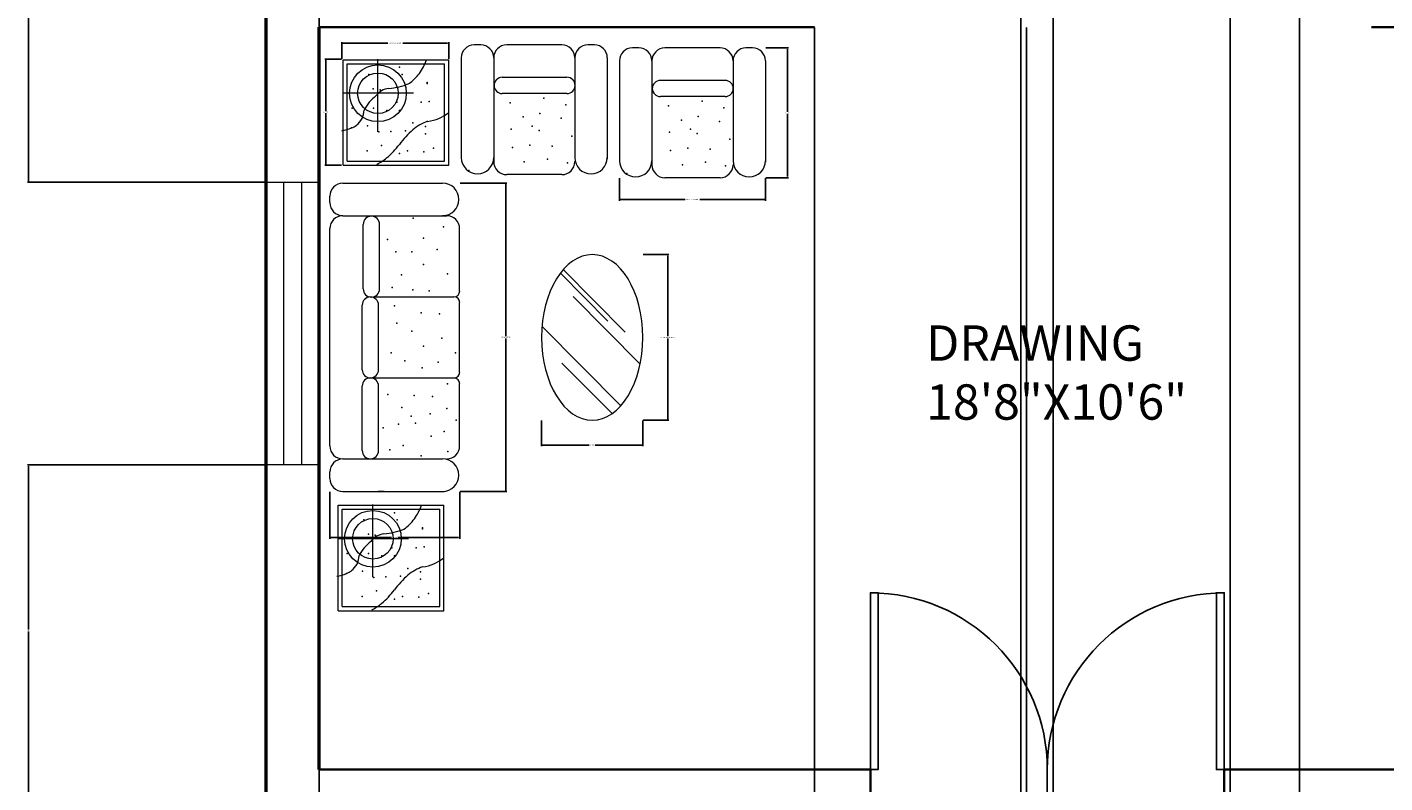
# Model space of a CAD drawing. Units: feet. Extents: x 2664 to 3060, y 1318 to 2005.
# Tile 3 of 5: x 2664 to 2894, y 1702 to 1830. Entities that reach past the tile are written whole.
import ezdxf

# ---------------------------------------------------------------- set-up
doc = ezdxf.new("R2010")
doc.units = ezdxf.units.FT
for name, color, linetype, lineweight in [('A-ANNO-DIMS', 2, 'Continuous', 18), ('A-AREA-IDEN', 109, 'Continuous', 18), ('A-WALL-EXTR', 130, 'Continuous', 50), ('DOOR', 249, 'Continuous', 25), ('FURNITURE', 240, 'Continuous', 13)]:
    doc.layers.add(name, color=color, linetype=linetype, lineweight=lineweight)
doc.layers.add('A-GLAZ', color=222, linetype='Continuous', lineweight=18, true_color=0xd4008b)
doc.layers.add('A-WALL-INTR', color=41, linetype='Continuous', lineweight=35, true_color=0xf5dd7a)
doc.styles.get("Standard").update_dxf_attribs({"font": 'arial.ttf'})
doc.dimstyles.get("Standard").update_dxf_attribs({"dimtxt": 0.18, "dimasz": 0.18, "dimexe": 0.18, "dimexo": 0.0625, "dimgap": 0.09, "dimtad": 0, "dimtih": 1, "dimtoh": 1, "dimdec": 4, "dimzin": 0, "dimdsep": 46, "dimtxsty": 'Standard', "dimcen": 0.09, "dimadec": 0, "dimazin": 0, "dimtfac": 1, "dimtdec": 4, "dimtofl": 0, "dimtmove": 0, "dimatfit": 3, "dimfxl": 1, "dimtolj": 1, "dimtzin": 0, "dimarcsym": 0})

# ---------------------------------------------------------------- blocks, each defined once
blk = doc.blocks.new('*U2')
for p, q in [((0, 0), (0, -6)), ((40, 0), (40, -6))]:
    blk.add_line(p, q)
blk.add_lwpolyline([(0, 0), (0, 40), (1.75, 40), (1.75, 0)], close=True)
blk.add_arc((0, 0), 40, 0, 90)
blk = doc.blocks.new('TABLE-END')
for p, q in [((-8.83, -9), (-8.83, 8.9)), ((-8.83, 8.9), (9.06, 8.9)), ((-8.14, -8.31), (-8.14, 8.21)), ((-8.14, 8.21), (8.38, 8.21)), ((-2.94, -3.32), (-2.94, 9)), ((8.38, -8.31), (8.38, 8.21)), ((9.06, -9), (9.06, 8.9)), ((3.1, 3.21), (-8.97, 3.21)), ((-8.83, -9), (9.06, -9)), ((-8.14, -8.31), (8.38, -8.31))]:
    blk.add_line(p, q)
for radius in [4.81, 3.44]:
    blk.add_circle((-2.94, 3.21), radius)
for centre, radius, start, end in [((-3.5, 11.98), 9.32, 324.6463, 340.6785), ((-2.19, 16.41), 12.41, 275.1129, 291.2782), ((-1.58, 10.62), 6.96, 304.0039, 324.6463), ((0.7, -2.61), 6.69, 126.4548, 153.626), ((-0.75, 0.94), 3.12, 96.1016, 144.1315), ((-8.44, 0.34), 3.14, 305.9664, 0.3439), ((-9.12, 1.28), 4.31, 293.3746, 305.9664), ((8.07, -8.93), 7.82, 109.24, 130.5005), ((4.71, 5.19), 6.79, 276.623, 309.8575), ((-9.98, 3.26), 6.46, 278.1279, 293.3746), ((12.46, -14.07), 14.57, 130.5005, 143.836), ((-9.43, 1.93), 12.54, 309.4558, 323.836), ((-7.51, -0.4), 9.52, 297.4626, 309.4558)]:
    blk.add_arc(centre, radius, start, end)
for p in [(0.71, 7.64), (-4.49, 6.42), (1.18, 6.4), (5.44, 5.05), (5.44, 4.89), (-3.72, 3.98), (-2.55, 3.81), (-7.32, 0.7), (-3.69, 0.7), (-1.43, 0.31), (0.25, 1.69), (0.71, 0.31), (4.37, 1.69), (5.75, 1.84), (3, -1.82), (-7.41, -2.67), (-4.73, -2.3), (-2.81, -3.35), (-0.75, -3.26), (1.74, -3.15), (5.12, -2.41), (5.14, -3.65), (-4.79, -6.56), (-2.35, -5.64), (2.08, -6.56), (4.83, -6.71), (6.51, -6.1), (0.72, -7.03)]:
    blk.add_point(p)
blk = doc.blocks.new('SOFA-3-SEAT')
for p, q in [((-11.01, -3.3), (-11.01, -2.2)), ((-8.81, 0), (8.12, 0)), ((-8.81, -5.51), (-4.95, -5.51)), ((-4.95, -5.51), (8.81, -5.51)), ((-11.01, -44.59), (-11.01, -7.71)), ((-5.34, -17.95), (-5.34, -6.98)), ((-2.59, -17.95), (-2.59, -6.98)), ((11.01, -18.31), (11.01, -7.71)), ((-5.51, -31.66), (-5.51, -20.69)), ((-3.58, -19.27), (10.05, -19.27)), ((-2.75, -31.66), (-2.75, -20.69)), ((11.01, -32.07), (11.01, -20.23)), ((-5.51, -45.38), (-5.51, -34.41)), ((-4.13, -33.03), (10.05, -33.03)), ((-2.75, -45.38), (-2.75, -34.41)), ((11.01, -44.59), (11.01, -34.04)), ((-8.81, -46.8), (8.12, -46.8)), ((-11.01, -50.1), (-11.01, -49)), ((-8.81, -52.3), (8.4, -52.3)), ((-2.79, -52.3), (-2.81, -52.3)), ((-1.79, -52.3), (-2.79, -52.3))]:
    blk.add_line(p, q)
for centre, radius, start, end in [((-8.81, -2.2), 2.2, 90, 180), ((8.12, -2.75), 2.75, 0, 90), ((-8.81, -3.3), 2.2, 180, 270), ((8.12, -2.75), 2.75, 270, 0), ((-8.81, -7.71), 2.2, 90, 180), ((-3.96, -6.98), 1.38, 90, 180), ((-3.96, -6.98), 1.38, 0, 90), ((8.81, -7.71), 2.2, 0, 90), ((-3.96, -17.95), 1.38, 180, 270), ((-3.96, -17.95), 1.38, 270, 0), ((10.05, -18.31), 0.963, 270, 0), ((-4.13, -20.69), 1.38, 90, 180), ((-4.13, -20.69), 1.38, 0, 90), ((10.05, -20.23), 0.963, 0, 90), ((-4.13, -31.66), 1.38, 180, 270), ((-4.13, -31.66), 1.38, 270, 0), ((10.05, -32.07), 0.963, 270, 0), ((-4.13, -34.41), 1.38, 90, 180), ((-4.13, -34.41), 1.38, 0, 90), ((10.05, -34.04), 0.963, 0, 90), ((-8.81, -44.59), 2.2, 180, 270), ((-4.13, -45.38), 1.38, 180, 270), ((-4.13, -45.38), 1.38, 270, 0), ((8.81, -44.59), 2.2, 270, 0), ((-8.81, -49), 2.2, 90, 180), ((8.12, -49.55), 2.75, 0, 90), ((-8.81, -50.1), 2.2, 180, 270), ((8.12, -49.55), 2.75, 270, 0), ((-2.76, -44.04), 8.26, 268.9725, 269.066), ((-2.75, -42.86), 9.44, 269.1265, 269.4492), ((-2.75, -44.04), 8.26, 269.411, 269.6618), ((-2.78, -44.04), 8.26, 269.9826, 270)]:
    blk.add_arc(centre, radius, start, end)
for p in [(3.15, -5.94), (8.25, -7.42), (-1.22, -9.57), (4.85, -9.35), (7.19, -11.26), (0.16, -11.65), (2.9, -11.65), (4.85, -13.8), (1.14, -15.55), (8.94, -15.36), (-0.42, -17.7), (3.09, -18.09), (5.82, -18.28), (-0.03, -20.82), (4.46, -21.98), (7.58, -22.18), (0.36, -23.74), (2.9, -25.1), (7.97, -26.27), (-0.62, -28.81), (4.85, -27.64), (10.31, -28.81), (1.73, -30.17), (4.65, -31.34), (7.38, -30.37), (8.94, -34.07), (-1.2, -35.83), (3.29, -36.02), (6.41, -36.22), (1.22, -38.06), (6.02, -39.14), (8.84, -38.21), (0.63, -40.87), (2.78, -39.55), (3.52, -40.73), (10.4, -40.21), (-1.96, -41.54), (6.18, -42.95), (8.4, -42.13), (-0.85, -45.24), (1.44, -44.5), (8.99, -45.54), (4.48, -46.28)]:
    blk.add_point(p)
blk = doc.blocks.new('TABLE-COFFEE-OVAL')
for p, q in [((2.67, 2.77), (-5.41, 10.92)), ((5.56, 0.91), (-4.93, 11.5)), ((8.13, -4.53), (-3.25, 6.96)), ((4.85, -11.6), (-8.51, 1.88)), ((3.36, -12.93), (-5.15, -4.35))]:
    blk.add_line(p, q)
at = {"extrusion": (0, 0, -1)}
blk.add_ellipse((0, 0), major_axis=(0, 14.05), ratio=0.611621, dxfattribs=at)
blk = doc.blocks.new('CHAIR-ARM')
for p, q in [((-9.08, 0), (-10.19, 0)), ((4.68, 0), (-4.68, 0)), ((10.19, 0), (9.08, 0)), ((-12.39, -2.2), (-12.39, -19.13)), ((-6.88, -2.2), (-6.88, -6.06)), ((-6.88, -2.2), (-6.88, -6.12)), ((-6.88, -2.2), (-6.88, -19.82)), ((6.88, -2.2), (6.88, -19.13)), ((12.39, -2.2), (12.39, -19.41)), ((5.54, -5.51), (-5.43, -5.51)), ((5.54, -8.26), (-5.43, -8.26)), ((4.68, -8.26), (-4.68, -8.26)), ((4.68, -22.02), (-4.68, -22.02))]:
    blk.add_line(p, q)
for centre, radius, start, end in [((-10.19, -2.2), 2.2, 90, 180), ((-9.08, -2.2), 2.2, 0, 90), ((-4.68, -2.2), 2.2, 90, 180), ((4.68, -2.2), 2.2, 0, 90), ((9.08, -2.2), 2.2, 90, 180), ((10.19, -2.2), 2.2, 0, 90), ((-5.43, -6.88), 1.38, 90, 180), ((-5.43, -6.88), 1.38, 180, 270), ((5.54, -6.88), 1.38, 0, 90), ((5.54, -6.88), 1.38, 270, 0), ((-9.63, -19.13), 2.75, 180, 270), ((-9.63, -19.13), 2.75, 270, 0), ((-4.68, -19.82), 2.2, 180, 270), ((4.68, -19.82), 2.2, 270, 0), ((9.63, -19.13), 2.75, 180, 270), ((9.63, -19.13), 2.75, 270, 0)]:
    blk.add_arc(centre, radius, start, end)
for p in [(1.63, -9.05), (-4.09, -9.81), (5.33, -10.16), (-1.86, -12.23), (-0.36, -13.79), (0.96, -11.64), (4.59, -12.46), (-3.89, -14.3), (0.81, -14.53), (6.36, -15.49), (-3.7, -17.42), (-0.77, -17.03), (3.03, -17.19), (-1.71, -19.86), (2.22, -19.41), (5.62, -20), (-11.11, -21.32)]:
    blk.add_point(p)
blk = doc.blocks.new('WINDOW-4FT')
for p, q in [((-24, 4.5), (24, 4.5)), ((-24, -4.5), (-24, 4.5)), ((24, 4.5), (24, -4.5)), ((-24, 1.5), (24, 1.5)), ((24, -1.5), (-24, -1.5)), ((24, -4.5), (-24, -4.5))]:
    blk.add_line(p, q)
blk = doc.blocks.new('*D20')
at = {"layer": 'A-ANNO-DIMS', "color": 0, "lineweight": -2, "transparency": 16777216}
for p, q in [((2717.13, 1824.69), (2717.13, 1827.53)), ((2717.31, 1827.35), (2724.94, 1827.35)), ((2735.08, 1827.35), (2727.45, 1827.35)), ((2735.26, 1824.69), (2735.26, 1827.53))]:
    blk.add_line(p, q, dxfattribs=at)
at = {"layer": 'A-ANNO-DIMS', "color": 0, "transparency": 16777216}
for points in [[(2717.31, 1827.38), (2717.31, 1827.32), (2717.13, 1827.35)], [(2735.08, 1827.38), (2735.08, 1827.32), (2735.26, 1827.35)]]:
    blk.add_solid(points, dxfattribs=at)
at = {"layer": 'Defpoints', "color": 0, "transparency": 16777216}
for p in [(2735.26, 1827.35), (2717.13, 1824.63), (2735.26, 1824.63)]:
    blk.add_point(p, dxfattribs=at)
at = {"layer": 'A-ANNO-DIMS', "color": 0, "transparency": 16777216, "insert": (2726.19, 1827.35), "char_height": 0.18, "attachment_point": 5}
blk.add_mtext('\\A1;END TABLE 18 TYP.', dxfattribs=at)
blk = doc.blocks.new('*D21')
at = {"layer": 'A-ANNO-DIMS', "color": 0, "lineweight": -2, "transparency": 16777216}
for p, q in [((2717.07, 1824.63), (2714.23, 1824.63)), ((2714.41, 1824.45), (2714.41, 1815.81)), ((2714.41, 1806.81), (2714.41, 1815.45)), ((2717.07, 1806.63), (2714.23, 1806.63))]:
    blk.add_line(p, q, dxfattribs=at)
at = {"layer": 'A-ANNO-DIMS', "color": 0, "transparency": 16777216}
for points in [[(2714.38, 1824.45), (2714.44, 1824.45), (2714.41, 1824.63)], [(2714.38, 1806.81), (2714.44, 1806.81), (2714.41, 1806.63)]]:
    blk.add_solid(points, dxfattribs=at)
at = {"layer": 'Defpoints', "color": 0, "transparency": 16777216}
for p in [(2714.41, 1824.63), (2717.13, 1824.63), (2717.13, 1806.63)]:
    blk.add_point(p, dxfattribs=at)
at = {"layer": 'A-ANNO-DIMS', "color": 0, "transparency": 16777216, "insert": (2714.41, 1815.63), "char_height": 0.18, "attachment_point": 5}
blk.add_mtext('\\A1;18 TYP.', dxfattribs=at)
blk = doc.blocks.new('*D22')
at = {"layer": 'A-ANNO-DIMS', "color": 0, "lineweight": -2, "transparency": 16777216}
for p, q in [((2764.21, 1804.45), (2764.21, 1800.62)), ((2788.99, 1804.45), (2788.99, 1800.62)), ((2764.39, 1800.8), (2775.36, 1800.8)), ((2788.81, 1800.8), (2777.84, 1800.8))]:
    blk.add_line(p, q, dxfattribs=at)
at = {"layer": 'A-ANNO-DIMS', "color": 0, "transparency": 16777216}
for points in [[(2764.39, 1800.83), (2764.39, 1800.77), (2764.21, 1800.8)], [(2788.81, 1800.83), (2788.81, 1800.77), (2788.99, 1800.8)]]:
    blk.add_solid(points, dxfattribs=at)
at = {"layer": 'Defpoints', "color": 0, "transparency": 16777216}
for p in [(2764.21, 1804.52), (2788.99, 1804.52), (2788.99, 1800.8)]:
    blk.add_point(p, dxfattribs=at)
at = {"layer": 'A-ANNO-DIMS', "color": 0, "transparency": 16777216, "insert": (2776.6, 1800.8), "char_height": 0.18, "attachment_point": 5}
blk.add_mtext('\\A1;ARMCHAIR 25 TYP.', dxfattribs=at)
blk = doc.blocks.new('*D23')
at = {"layer": 'A-ANNO-DIMS', "color": 0, "lineweight": -2, "transparency": 16777216}
for p, q in [((2789.05, 1826.54), (2792.88, 1826.54)), ((2792.7, 1826.36), (2792.7, 1815.71)), ((2792.7, 1804.7), (2792.7, 1815.35)), ((2789.05, 1804.52), (2792.88, 1804.52))]:
    blk.add_line(p, q, dxfattribs=at)
at = {"layer": 'A-ANNO-DIMS', "color": 0, "transparency": 16777216}
for points in [[(2792.67, 1826.36), (2792.73, 1826.36), (2792.7, 1826.54)], [(2792.67, 1804.7), (2792.73, 1804.7), (2792.7, 1804.52)]]:
    blk.add_solid(points, dxfattribs=at)
at = {"layer": 'Defpoints', "color": 0, "transparency": 16777216}
for p in [(2788.99, 1826.54), (2792.7, 1826.54), (2788.99, 1804.52)]:
    blk.add_point(p, dxfattribs=at)
at = {"layer": 'A-ANNO-DIMS', "color": 0, "transparency": 16777216, "insert": (2792.7, 1815.53), "char_height": 0.18, "attachment_point": 5}
blk.add_mtext('\\A1;22 TYP.', dxfattribs=at)
blk = doc.blocks.new('*D26')
at = {"layer": 'A-ANNO-DIMS', "color": 0, "lineweight": -2, "transparency": 16777216}
for p, q in [((2737.18, 1803.58), (2745.14, 1803.58)), ((2744.96, 1803.4), (2744.96, 1777.62)), ((2744.96, 1751.46), (2744.96, 1777.25)), ((2737.18, 1751.28), (2745.14, 1751.28))]:
    blk.add_line(p, q, dxfattribs=at)
at = {"layer": 'A-ANNO-DIMS', "color": 0, "transparency": 16777216}
for points in [[(2744.93, 1803.4), (2744.99, 1803.4), (2744.96, 1803.58)], [(2744.93, 1751.46), (2744.99, 1751.46), (2744.96, 1751.28)]]:
    blk.add_solid(points, dxfattribs=at)
at = {"layer": 'Defpoints', "color": 0, "transparency": 16777216}
for p in [(2737.12, 1803.58), (2744.96, 1803.58), (2737.12, 1751.28)]:
    blk.add_point(p, dxfattribs=at)
at = {"layer": 'A-ANNO-DIMS', "color": 0, "transparency": 16777216, "insert": (2744.96, 1777.43), "char_height": 0.18, "attachment_point": 5}
blk.add_mtext('\\A1;SOFA 52 TYP.', dxfattribs=at)
blk = doc.blocks.new('*D27')
at = {"layer": 'A-ANNO-DIMS', "color": 0, "lineweight": -2, "transparency": 16777216}
for p, q in [((2715.1, 1751.22), (2715.1, 1743.26)), ((2737.12, 1751.22), (2737.12, 1743.26)), ((2715.28, 1743.44), (2725.58, 1743.44)), ((2736.94, 1743.44), (2726.64, 1743.44))]:
    blk.add_line(p, q, dxfattribs=at)
at = {"layer": 'A-ANNO-DIMS', "color": 0, "transparency": 16777216}
for points in [[(2715.28, 1743.47), (2715.28, 1743.41), (2715.1, 1743.44)], [(2736.94, 1743.47), (2736.94, 1743.41), (2737.12, 1743.44)]]:
    blk.add_solid(points, dxfattribs=at)
at = {"layer": 'Defpoints', "color": 0, "transparency": 16777216}
for p in [(2715.1, 1751.28), (2737.12, 1751.28), (2737.12, 1743.44)]:
    blk.add_point(p, dxfattribs=at)
at = {"layer": 'A-ANNO-DIMS', "color": 0, "transparency": 16777216, "insert": (2726.11, 1743.44), "char_height": 0.18, "attachment_point": 5}
blk.add_mtext('\\A1;22 TYP.', dxfattribs=at)
blk = doc.blocks.new('*D28')
at = {"layer": 'A-ANNO-DIMS', "color": 0, "lineweight": -2, "transparency": 16777216}
for p, q in [((2768.26, 1791.46), (2772.59, 1791.46)), ((2772.41, 1791.28), (2772.41, 1777.6)), ((2772.41, 1763.55), (2772.41, 1777.23)), ((2768.26, 1763.37), (2772.59, 1763.37))]:
    blk.add_line(p, q, dxfattribs=at)
at = {"layer": 'A-ANNO-DIMS', "color": 0, "transparency": 16777216}
for points in [[(2772.38, 1791.28), (2772.44, 1791.28), (2772.41, 1791.46)], [(2772.38, 1763.55), (2772.44, 1763.55), (2772.41, 1763.37)]]:
    blk.add_solid(points, dxfattribs=at)
at = {"layer": 'Defpoints', "color": 0, "transparency": 16777216}
for p in [(2768.19, 1791.46), (2772.41, 1791.46), (2768.19, 1763.37)]:
    blk.add_point(p, dxfattribs=at)
at = {"layer": 'A-ANNO-DIMS', "color": 0, "transparency": 16777216, "insert": (2772.41, 1777.42), "char_height": 0.18, "attachment_point": 5}
blk.add_mtext('\\A1;COFFEE TABLE 28 TYP.', dxfattribs=at)
blk = doc.blocks.new('*D29')
at = {"layer": 'A-ANNO-DIMS', "color": 0, "lineweight": -2, "transparency": 16777216}
for p, q in [((2751.01, 1763.3), (2751.01, 1758.97)), ((2768.19, 1763.3), (2768.19, 1758.97)), ((2751.19, 1759.15), (2759.08, 1759.15)), ((2768.01, 1759.15), (2760.12, 1759.15))]:
    blk.add_line(p, q, dxfattribs=at)
at = {"layer": 'A-ANNO-DIMS', "color": 0, "transparency": 16777216}
for points in [[(2751.19, 1759.18), (2751.19, 1759.12), (2751.01, 1759.15)], [(2768.01, 1759.18), (2768.01, 1759.12), (2768.19, 1759.15)]]:
    blk.add_solid(points, dxfattribs=at)
at = {"layer": 'Defpoints', "color": 0, "transparency": 16777216}
for p in [(2751.01, 1763.37), (2768.19, 1763.37), (2768.19, 1759.15)]:
    blk.add_point(p, dxfattribs=at)
at = {"layer": 'A-ANNO-DIMS', "color": 0, "transparency": 16777216, "insert": (2759.6, 1759.15), "char_height": 0.18, "attachment_point": 5}
blk.add_mtext('\\A1;17 TYP.', dxfattribs=at)
blk = doc.blocks.new('*D41')
at = {"layer": 'A-ANNO-DIMS', "color": 0, "lineweight": -2, "transparency": 16777216}
for p, q in [((2704.22, 1875.57), (2663.82, 1875.57)), ((2664, 1875.39), (2664, 1839.85)), ((2664, 1803.95), (2664, 1839.49)), ((2704.22, 1803.77), (2663.82, 1803.77))]:
    blk.add_line(p, q, dxfattribs=at)
at = {"layer": 'A-ANNO-DIMS', "color": 0, "transparency": 16777216}
for points in [[(2663.97, 1875.39), (2664.03, 1875.39), (2664, 1875.57)], [(2663.97, 1803.95), (2664.03, 1803.95), (2664, 1803.77)]]:
    blk.add_solid(points, dxfattribs=at)
at = {"layer": 'Defpoints', "color": 0, "transparency": 16777216}
for p in [(2704.28, 1875.57), (2664, 1803.77), (2704.28, 1803.77)]:
    blk.add_point(p, dxfattribs=at)
at = {"layer": 'A-ANNO-DIMS', "color": 0, "transparency": 16777216, "insert": (2664, 1839.67), "char_height": 0.18, "attachment_point": 5}
blk.add_mtext('\\A1;71.8', dxfattribs=at)
blk = doc.blocks.new('*D42')
at = {"layer": 'A-ANNO-DIMS', "color": 0, "lineweight": -2, "transparency": 16777216}
for p, q in [((2704.22, 1755.77), (2663.82, 1755.77)), ((2664, 1755.59), (2664, 1727.85)), ((2664, 1699.75), (2664, 1727.49)), ((2704.22, 1699.57), (2663.82, 1699.57))]:
    blk.add_line(p, q, dxfattribs=at)
at = {"layer": 'A-ANNO-DIMS', "color": 0, "transparency": 16777216}
for points in [[(2663.97, 1755.59), (2664.03, 1755.59), (2664, 1755.77)], [(2663.97, 1699.75), (2664.03, 1699.75), (2664, 1699.57)]]:
    blk.add_solid(points, dxfattribs=at)
at = {"layer": 'Defpoints', "color": 0, "transparency": 16777216}
for p in [(2704.28, 1755.77), (2664, 1699.57), (2704.28, 1699.57)]:
    blk.add_point(p, dxfattribs=at)
at = {"layer": 'A-ANNO-DIMS', "color": 0, "transparency": 16777216, "insert": (2664, 1727.67), "char_height": 0.18, "attachment_point": 5}
blk.add_mtext('\\A1;56.2', dxfattribs=at)
blk = doc.blocks.new('*D48')
at = {"layer": 'A-ANNO-DIMS', "color": 0, "lineweight": -2, "transparency": 16777216}
for p, q in [((2879.53, 1619.63), (2879.53, 2005.03)), ((2879.71, 2004.85), (2929.25, 2004.85)), ((2979.35, 2004.85), (2929.81, 2004.85)), ((2979.53, 1619.63), (2979.53, 2005.03))]:
    blk.add_line(p, q, dxfattribs=at)
at = {"layer": 'A-ANNO-DIMS', "color": 0, "transparency": 16777216}
for points in [[(2879.71, 2004.88), (2879.71, 2004.82), (2879.53, 2004.85)], [(2979.35, 2004.88), (2979.35, 2004.82), (2979.53, 2004.85)]]:
    blk.add_solid(points, dxfattribs=at)
at = {"layer": 'Defpoints', "color": 0, "transparency": 16777216}
for p in [(2979.53, 2004.85), (2879.53, 1619.57), (2979.53, 1619.57)]:
    blk.add_point(p, dxfattribs=at)
at = {"layer": 'A-ANNO-DIMS', "color": 0, "transparency": 16777216, "insert": (2929.53, 2004.85), "char_height": 0.18, "attachment_point": 5}
blk.add_mtext('\\A1;100', dxfattribs=at)
blk = doc.blocks.new('*D53')
at = {"layer": 'A-ANNO-DIMS', "color": 0, "lineweight": -2, "transparency": 16777216}
for p, q in [((2797.28, 1830.01), (2797.28, 1318.11)), ((2833.28, 1830.01), (2833.28, 1318.11)), ((2797.46, 1318.29), (2815.06, 1318.29)), ((2833.1, 1318.29), (2815.5, 1318.29))]:
    blk.add_line(p, q, dxfattribs=at)
at = {"layer": 'A-ANNO-DIMS', "color": 0, "transparency": 16777216}
for points in [[(2797.46, 1318.32), (2797.46, 1318.26), (2797.28, 1318.29)], [(2833.1, 1318.32), (2833.1, 1318.26), (2833.28, 1318.29)]]:
    blk.add_solid(points, dxfattribs=at)
at = {"layer": 'Defpoints', "color": 0, "transparency": 16777216}
for p in [(2797.28, 1830.07), (2833.28, 1830.07), (2833.28, 1318.29)]:
    blk.add_point(p, dxfattribs=at)
at = {"layer": 'A-ANNO-DIMS', "color": 0, "transparency": 16777216, "insert": (2815.28, 1318.29), "char_height": 0.18, "attachment_point": 5}
blk.add_mtext('\\A1;36', dxfattribs=at)
blk = doc.blocks.new('*D54')
at = {"layer": 'A-ANNO-DIMS', "color": 0, "lineweight": -2, "transparency": 16777216}
for p, q in [((2837.78, 1868.51), (2837.78, 1318.11)), ((2867.78, 1868.51), (2867.78, 1318.11)), ((2837.96, 1318.29), (2852.56, 1318.29)), ((2867.6, 1318.29), (2853, 1318.29))]:
    blk.add_line(p, q, dxfattribs=at)
at = {"layer": 'A-ANNO-DIMS', "color": 0, "transparency": 16777216}
for points in [[(2837.96, 1318.32), (2837.96, 1318.26), (2837.78, 1318.29)], [(2867.6, 1318.32), (2867.6, 1318.26), (2867.78, 1318.29)]]:
    blk.add_solid(points, dxfattribs=at)
at = {"layer": 'Defpoints', "color": 0, "transparency": 16777216}
for p in [(2837.78, 1868.57), (2867.78, 1868.57), (2867.78, 1318.29)]:
    blk.add_point(p, dxfattribs=at)
at = {"layer": 'A-ANNO-DIMS', "color": 0, "transparency": 16777216, "insert": (2852.78, 1318.29), "char_height": 0.18, "attachment_point": 5}
blk.add_mtext('\\A1;30', dxfattribs=at)
blk = doc.blocks.new('*D55')
at = {"layer": 'A-ANNO-DIMS', "color": 0, "lineweight": -2, "transparency": 16777216}
for p, q in [((2833.28, 1830.01), (2833.28, 1318.11)), ((2837.78, 1830.01), (2837.78, 1318.11)), ((2833.46, 1318.29), (2835.27, 1318.29)), ((2837.6, 1318.29), (2835.79, 1318.29))]:
    blk.add_line(p, q, dxfattribs=at)
at = {"layer": 'A-ANNO-DIMS', "color": 0, "transparency": 16777216}
for points in [[(2833.46, 1318.32), (2833.46, 1318.26), (2833.28, 1318.29)], [(2837.6, 1318.32), (2837.6, 1318.26), (2837.78, 1318.29)]]:
    blk.add_solid(points, dxfattribs=at)
at = {"layer": 'Defpoints', "color": 0, "transparency": 16777216}
for p in [(2833.28, 1830.07), (2837.78, 1830.07), (2837.78, 1318.29)]:
    blk.add_point(p, dxfattribs=at)
at = {"layer": 'A-ANNO-DIMS', "color": 0, "transparency": 16777216, "insert": (2835.53, 1318.29), "char_height": 0.18, "attachment_point": 5}
blk.add_mtext('\\A1;4.5', dxfattribs=at)
blk = doc.blocks.new('*D59')
at = {"layer": 'A-ANNO-DIMS', "color": 0, "lineweight": -2, "transparency": 16777216}
for p, q in [((2713.28, 1488.63), (2713.28, 2005.03)), ((2713.46, 2004.85), (2772.5, 2004.85)), ((2832.1, 2004.85), (2773.06, 2004.85)), ((2832.28, 1489.53), (2832.28, 2005.03))]:
    blk.add_line(p, q, dxfattribs=at)
at = {"layer": 'A-ANNO-DIMS', "color": 0, "transparency": 16777216}
for points in [[(2713.46, 2004.88), (2713.46, 2004.82), (2713.28, 2004.85)], [(2832.1, 2004.88), (2832.1, 2004.82), (2832.28, 2004.85)]]:
    blk.add_solid(points, dxfattribs=at)
at = {"layer": 'Defpoints', "color": 0, "transparency": 16777216}
for p in [(2832.28, 2004.85), (2713.28, 1488.57), (2832.28, 1489.47)]:
    blk.add_point(p, dxfattribs=at)
at = {"layer": 'A-ANNO-DIMS', "color": 0, "transparency": 16777216, "insert": (2772.78, 2004.85), "char_height": 0.18, "attachment_point": 5}
blk.add_mtext('\\A1;119', dxfattribs=at)

msp = doc.modelspace()

# ---------------------------------------------------------------- linework, layer by layer
at = {"layer": 'A-WALL-EXTR'}
for p, q in [((2704.28, 1349.571), (2704.28, 1973.571)), ((2713.28, 1704.071), (2713.28, 1830.071))]:
    msp.add_line(p, q, dxfattribs=at)
at = {"layer": 'A-WALL-INTR'}
for p, q in [((2713.28, 1830.071), (2797.28, 1830.071)), ((2891.78, 1830.071), (2896.28, 1830.071)), ((2713.28, 1704.071), (2806.78, 1704.071)), ((2806.78, 1699.571), (2806.78, 1704.071)), ((2866.78, 1699.571), (2866.78, 1704.071)), ((2866.78, 1704.071), (2936.78, 1704.071))]:
    msp.add_line(p, q, dxfattribs=at)

# ---------------------------------------------------------------- block references
at = {"layer": 'A-GLAZ', "rotation": 89.99999999999957}
msp.add_blockref('WINDOW-4FT', (2708.78, 1779.772), dxfattribs=at)
at = {"layer": 'DOOR', "yscale": 0.7500000000000038, "zscale": 0.7500000000000038}
for p, xscale in [((2806.78, 1704.071), 0.7500000000000038), ((2866.78, 1704.071), -0.7500000000000038)]:
    msp.add_blockref('*U2', p, dxfattribs=dict(at, xscale=xscale))
at = {"layer": 'FURNITURE'}
for name, p in [('CHAIR-ARM', (2749.769, 1827.061)), ('CHAIR-ARM', (2776.599, 1826.538)), ('TABLE-END', (2726.193, 1815.632)), ('SOFA-3-SEAT', (2726.106, 1803.584)), ('TABLE-COFFEE-OVAL', (2759.601, 1777.415)), ('TABLE-END', (2725.347, 1740.034))]:
    msp.add_blockref(name, p, dxfattribs=at)

# ---------------------------------------------------------------- texts
at = {"layer": 'A-AREA-IDEN', "insert": (2816.227, 1779.457), "char_height": 6, "attachment_point": 1}
msp.add_mtext_dynamic_manual_height_columns('DRAWING \\P18\'8"X10\'6"', width=22.955, gutter_width=12.5, heights=[0], dxfattribs=at)

# ---------------------------------------------------------------- dimensions: what is measured, and where the dimension line sits
at = {"layer": 'A-ANNO-DIMS'}
for base, p1, p2, override, picture, middle in [((2832.28, 2004.851), (2713.28, 1488.571), (2832.28, 1489.471), {"dimdec": 0, "dimlfac": 1, "dimrnd": 0, "dimzin": 0, "dimdsep": 46, "dimlunit": 2}, '*D59', (2772.78, 2004.851)), ((2979.53, 2004.851), (2879.53, 1619.571), (2979.53, 1619.571), {"dimdec": 0, "dimlfac": 1, "dimrnd": 0, "dimzin": 0, "dimdsep": 46, "dimlunit": 2}, '*D48', (2929.53, 2004.851)), ((2867.78, 1318.291), (2837.78, 1868.571), (2867.78, 1868.571), {"dimdec": 0, "dimlfac": 1, "dimrnd": 0, "dimzin": 0, "dimdsep": 46, "dimlunit": 2}, '*D54', (2852.78, 1318.291)), ((2833.28, 1318.291), (2797.28, 1830.071), (2833.28, 1830.071), {"dimdec": 0, "dimlfac": 1, "dimrnd": 0, "dimzin": 0, "dimdsep": 46, "dimlunit": 2}, '*D53', (2815.28, 1318.291)), ((2837.78, 1318.291), (2833.28, 1830.071), (2837.78, 1830.071), {"dimdec": 1, "dimlfac": 1, "dimrnd": 0, "dimzin": 0, "dimdsep": 46, "dimlunit": 2}, '*D55', (2835.53, 1318.291))]:
    dim = msp.add_linear_dim(base=base, p1=p1, p2=p2, dimstyle='Standard', override=override, dxfattribs=at)
    dim.commit()
    dim.dimension.update_dxf_attribs({"geometry": picture, "text_midpoint": middle})
for base, p1, p2, picture, middle in [((2664, 1803.772), (2704.28, 1875.571), (2704.28, 1803.772), '*D41', (2664, 1839.671)), ((2664, 1699.571), (2704.28, 1755.772), (2704.28, 1699.571), '*D42', (2664, 1727.671))]:
    dim = msp.add_linear_dim(base=base, p1=p1, p2=p2, angle=90, dimstyle='Standard', override={"dimdec": 1, "dimlfac": 1, "dimrnd": 0, "dimzin": 0, "dimdsep": 46, "dimlunit": 2}, dxfattribs=at)
    dim.commit()
    dim.dimension.update_dxf_attribs({"geometry": picture, "text_midpoint": middle})
for base, p1, p2, text, picture, middle in [((2735.257, 1827.348), (2717.13, 1824.629), (2735.257, 1824.629), 'END TABLE <> TYP.', '*D20', (2726.193, 1827.348)), ((2788.987, 1800.8), (2764.212, 1804.516), (2788.987, 1804.516), 'ARMCHAIR <> TYP.', '*D22', (2776.599, 1800.8)), ((2768.193, 1759.153), (2751.009, 1763.367), (2768.193, 1763.367), '<> TYP.', '*D29', (2759.601, 1759.153)), ((2737.117, 1743.436), (2715.096, 1751.282), (2737.117, 1751.282), '<> TYP.', '*D27', (2726.106, 1743.436))]:
    dim = msp.add_linear_dim(base=base, p1=p1, p2=p2, text=text, dimstyle='Standard', override={"dimdec": 0, "dimlfac": 1, "dimrnd": 0, "dimzin": 0, "dimdsep": 46, "dimlunit": 2}, dxfattribs=at)
    dim.commit()
    dim.dimension.update_dxf_attribs({"geometry": picture, "text_midpoint": middle})
for base, p1, p2, text, picture, middle in [((2792.703, 1826.538), (2788.987, 1804.516), (2788.987, 1826.538), '<> TYP.', '*D23', (2792.703, 1815.527)), ((2714.411, 1824.629), (2717.13, 1806.635), (2717.13, 1824.629), '<> TYP.', '*D21', (2714.411, 1815.632)), ((2744.963, 1803.584), (2737.117, 1751.282), (2737.117, 1803.584), 'SOFA <> TYP.', '*D26', (2744.963, 1777.433)), ((2772.408, 1791.464), (2768.193, 1763.367), (2768.193, 1791.464), 'COFFEE TABLE <> TYP.', '*D28', (2772.408, 1777.415))]:
    dim = msp.add_linear_dim(base=base, p1=p1, p2=p2, angle=90, text=text, dimstyle='Standard', override={"dimdec": 0, "dimlfac": 1, "dimrnd": 0, "dimzin": 0, "dimdsep": 46, "dimlunit": 2}, dxfattribs=at)
    dim.commit()
    dim.dimension.update_dxf_attribs({"geometry": picture, "text_midpoint": middle})

doc.saveas('drawing.dxf')
